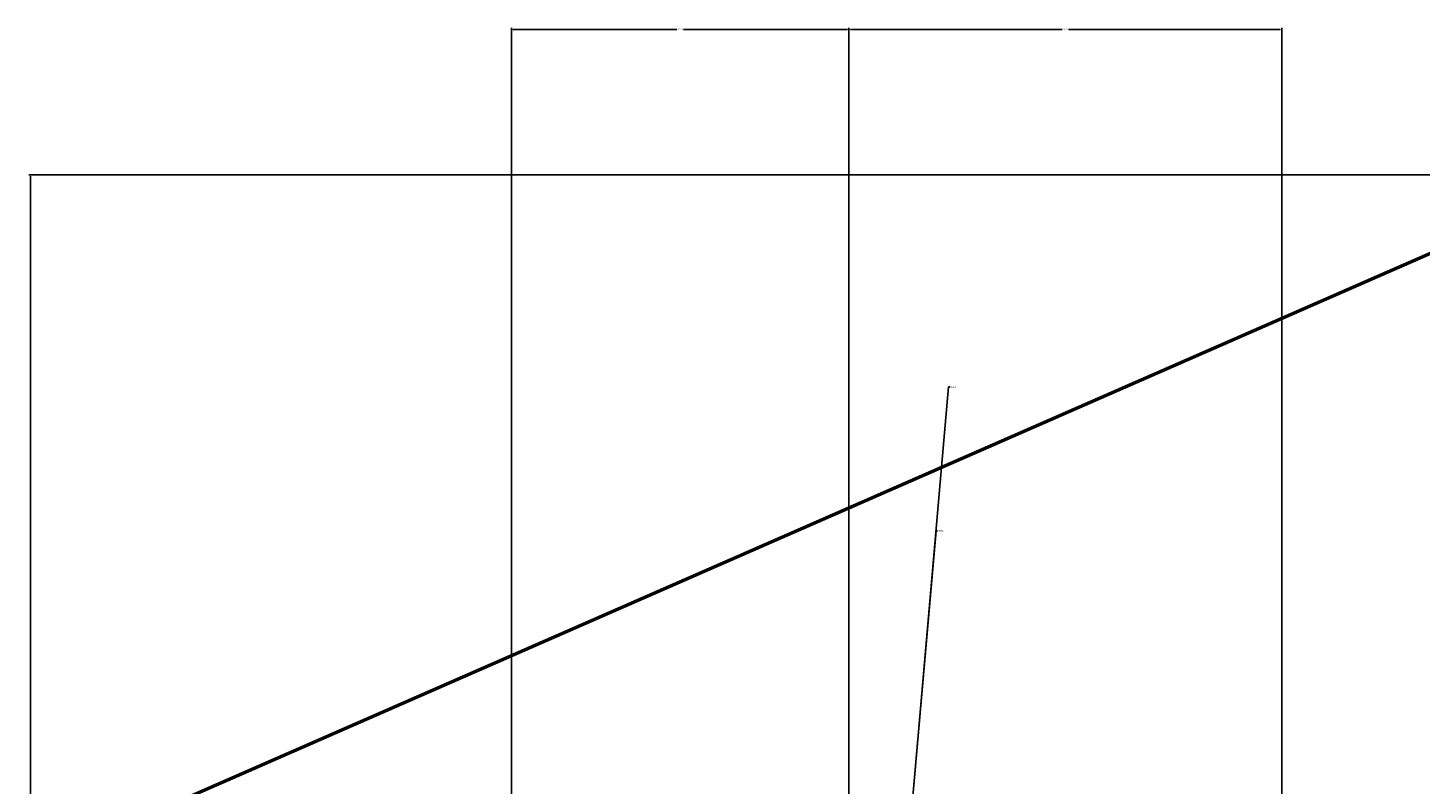
# Model space of a CAD drawing. Units: inches. Extents: x 457 to 775, y 319 to 541.
# Tile 7 of 12: x 457 to 623, y 450 to 541. Entities that reach past the tile are written whole.
import ezdxf

# ---------------------------------------------------------------- set-up
doc = ezdxf.new("R2010")
doc.units = ezdxf.units.IN
doc.header["$MEASUREMENT"] = 0
doc.layers.add('M-DIMS', color=2, linetype='Continuous', lineweight=18)
doc.layers.add('M-OUTL', color=7, linetype='Continuous', lineweight=50)
doc.styles.get("Standard").update_dxf_attribs({"font": 'arial.ttf'})
doc.dimstyles.get("Standard").update_dxf_attribs({"dimtxt": 0.18, "dimasz": 0.18, "dimexe": 0.18, "dimexo": 0.0625, "dimgap": 0.09, "dimtad": 0, "dimtih": 1, "dimtoh": 1, "dimdec": 4, "dimzin": 0, "dimdsep": 46, "dimtxsty": 'Standard', "dimcen": 0.09, "dimadec": 0, "dimazin": 0, "dimtfac": 1, "dimtdec": 4, "dimtofl": 0, "dimtmove": 0, "dimatfit": 3, "dimfxl": 1, "dimtolj": 1, "dimtzin": 0, "dimarcsym": 0})

# ---------------------------------------------------------------- blocks, each defined once
blk = doc.blocks.new('*D3')
at = {"layer": 'Defpoints', "color": 0, "transparency": 16777216}
for p in [(456.91, 523.21), (646, 523.21), (474.31, 336.7)]:
    blk.add_point(p, dxfattribs=at)
at = {"layer": 'M-DIMS', "color": 0, "lineweight": -2, "transparency": 16777216}
for p, q in [((645.94, 523.21), (456.73, 523.21)), ((456.91, 523.03), (456.91, 430.14)), ((456.91, 336.88), (456.91, 429.77)), ((474.24, 336.7), (456.73, 336.7))]:
    blk.add_line(p, q, dxfattribs=at)
at = {"layer": 'M-DIMS', "color": 0, "transparency": 16777216}
for points in [[(456.88, 523.03), (456.94, 523.03), (456.91, 523.21)], [(456.88, 336.88), (456.94, 336.88), (456.91, 336.7)]]:
    blk.add_solid(points, dxfattribs=at)
at = {"layer": 'M-DIMS', "color": 0, "transparency": 16777216, "insert": (456.91, 429.95), "char_height": 0.18, "attachment_point": 5}
blk.add_mtext('\\A1;186.5', dxfattribs=at)
blk = doc.blocks.new('*D16')
at = {"layer": 'Defpoints', "color": 0, "transparency": 16777216}
for p in [(554.93, 540.61), (514.5, 430.73), (554.93, 361.7)]:
    blk.add_point(p, dxfattribs=at)
at = {"layer": 'M-DIMS', "color": 0, "lineweight": -2, "transparency": 16777216}
for p, q in [((514.5, 430.79), (514.5, 540.79)), ((514.68, 540.61), (534.32, 540.61)), ((554.75, 540.61), (535.11, 540.61)), ((554.93, 361.76), (554.93, 540.79))]:
    blk.add_line(p, q, dxfattribs=at)
at = {"layer": 'M-DIMS', "color": 0, "transparency": 16777216}
for points in [[(514.68, 540.64), (514.68, 540.58), (514.5, 540.61)], [(554.75, 540.64), (554.75, 540.58), (554.93, 540.61)]]:
    blk.add_solid(points, dxfattribs=at)
at = {"layer": 'M-DIMS', "color": 0, "transparency": 16777216, "insert": (534.72, 540.61), "char_height": 0.18, "attachment_point": 5}
blk.add_mtext('\\A1;40.43', dxfattribs=at)
blk = doc.blocks.new('*D17')
at = {"layer": 'Defpoints', "color": 0, "transparency": 16777216}
for p in [(606.76, 540.61), (606.76, 422.64), (554.93, 361.7)]:
    blk.add_point(p, dxfattribs=at)
at = {"layer": 'M-DIMS', "color": 0, "lineweight": -2, "transparency": 16777216}
for p, q in [((554.93, 361.76), (554.93, 540.79)), ((555.11, 540.61), (580.45, 540.61)), ((606.58, 540.61), (581.24, 540.61)), ((606.76, 422.7), (606.76, 540.79))]:
    blk.add_line(p, q, dxfattribs=at)
at = {"layer": 'M-DIMS', "color": 0, "transparency": 16777216}
for points in [[(555.11, 540.64), (555.11, 540.58), (554.93, 540.61)], [(606.58, 540.64), (606.58, 540.58), (606.76, 540.61)]]:
    blk.add_solid(points, dxfattribs=at)
at = {"layer": 'M-DIMS', "color": 0, "transparency": 16777216, "insert": (580.85, 540.61), "char_height": 0.18, "attachment_point": 5}
blk.add_mtext('\\A1;51.83', dxfattribs=at)
blk = doc.blocks.new('*D19')
at = {"layer": 'Defpoints', "color": 0, "transparency": 16777216}
for p in [(562.39, 446.77), (554.93, 361.7)]:
    blk.add_point(p, dxfattribs=at)
at = {"layer": 'M-DIMS', "color": 0, "lineweight": -2, "transparency": 16777216}
for p, q in [((566.87, 497.81), (562.41, 446.95)), ((567.05, 497.81), (566.87, 497.81)), ((554.84, 361.7), (555.02, 361.7)), ((554.93, 361.61), (554.93, 361.79))]:
    blk.add_line(p, q, dxfattribs=at)
at = {"layer": 'M-DIMS', "color": 0, "transparency": 16777216}
blk.add_solid([(562.38, 446.95), (562.44, 446.95), (562.39, 446.77)], dxfattribs=at)
at = {"layer": 'M-DIMS', "color": 0, "transparency": 16777216, "insert": (567.46, 497.81), "char_height": 0.18, "attachment_point": 5}
blk.add_mtext('\\A1;R85.4', dxfattribs=at)
blk = doc.blocks.new('*D20')
at = {"layer": 'Defpoints', "color": 0, "transparency": 16777216}
for p in [(561.45, 436.01), (554.93, 361.7)]:
    blk.add_point(p, dxfattribs=at)
at = {"layer": 'M-DIMS', "color": 0, "lineweight": -2, "transparency": 16777216}
for p, q in [((565.36, 480.6), (561.47, 436.19)), ((565.54, 480.6), (565.36, 480.6)), ((554.84, 361.7), (555.02, 361.7)), ((554.93, 361.61), (554.93, 361.79))]:
    blk.add_line(p, q, dxfattribs=at)
at = {"layer": 'M-DIMS', "color": 0, "transparency": 16777216}
blk.add_solid([(561.44, 436.19), (561.5, 436.19), (561.45, 436.01)], dxfattribs=at)
at = {"layer": 'M-DIMS', "color": 0, "transparency": 16777216, "insert": (565.95, 480.6), "char_height": 0.18, "attachment_point": 5}
blk.add_mtext('\\A1;R74.6', dxfattribs=at)

msp = doc.modelspace()

# ---------------------------------------------------------------- linework, layer by layer
at = {"layer": 'M-OUTL'}
msp.add_line((474.306, 448.059), (646.001, 523.213), dxfattribs=at)

# ---------------------------------------------------------------- dimensions: what is measured, and where the dimension line sits
at = {"layer": 'M-DIMS'}
for base, p1, p2, picture, middle in [((554.931, 540.613), (514.502, 430.729), (554.931, 361.696), '*D16', (534.716, 540.613)), ((606.761, 540.613), (554.931, 361.696), (606.761, 422.636), '*D17', (580.846, 540.613))]:
    dim = msp.add_linear_dim(base=base, p1=p1, p2=p2, dimstyle='Standard', override={"dimdec": 2, "dimlfac": 1, "dimrnd": 0, "dimzin": 0, "dimdsep": 46, "dimlunit": 2}, dxfattribs=at)
    dim.commit()
    dim.dimension.update_dxf_attribs({"geometry": picture, "text_midpoint": middle})
dim = msp.add_linear_dim(base=(456.906, 523.213), p1=(474.306, 336.696), p2=(646.001, 523.213), angle=90, dimstyle='Standard', override={"dimdec": 1, "dimlfac": 1, "dimrnd": 0, "dimzin": 0, "dimdsep": 46, "dimlunit": 2}, dxfattribs=at)
dim.commit()
dim.dimension.update_dxf_attribs({"geometry": '*D3', "text_midpoint": (456.906, 429.954)})
for mpoint, picture, middle in [((562.393, 446.769), '*D19', (567.46, 497.813)), ((561.45, 436.011), '*D20', (565.951, 480.599))]:
    dim = msp.add_radius_dim(center=(554.931, 361.696), mpoint=mpoint, dimstyle='Standard', override={"dimdec": 1, "dimlfac": 1, "dimrnd": 0, "dimzin": 0, "dimdsep": 46, "dimlunit": 2}, dxfattribs=at)
    dim.commit()
    dim.dimension.update_dxf_attribs({"geometry": picture, "text_midpoint": middle, "dimtype": 164})

doc.saveas('drawing.dxf')
